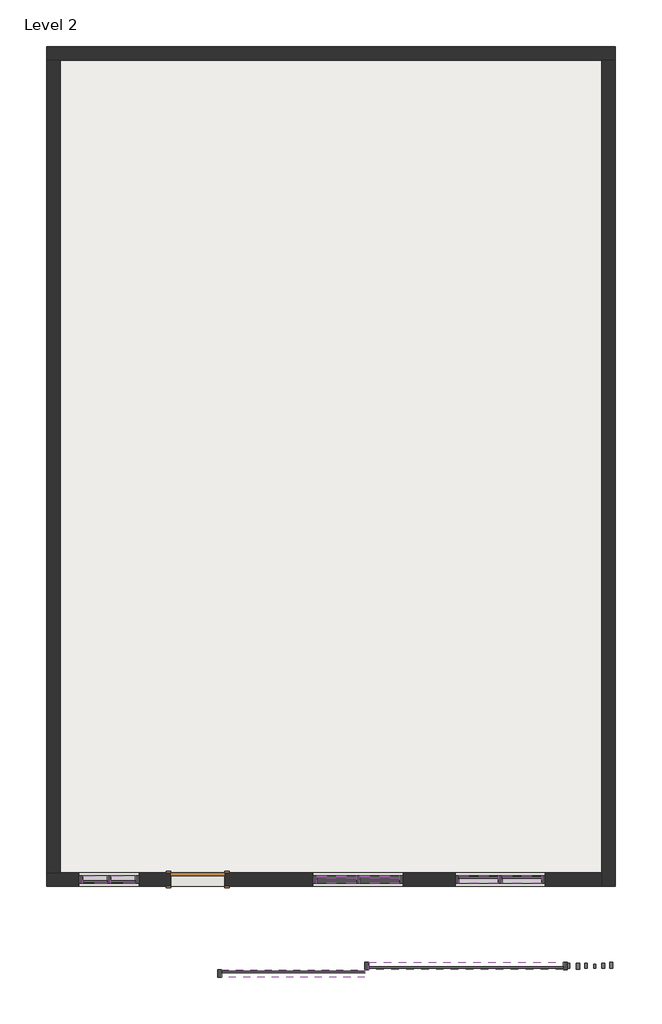
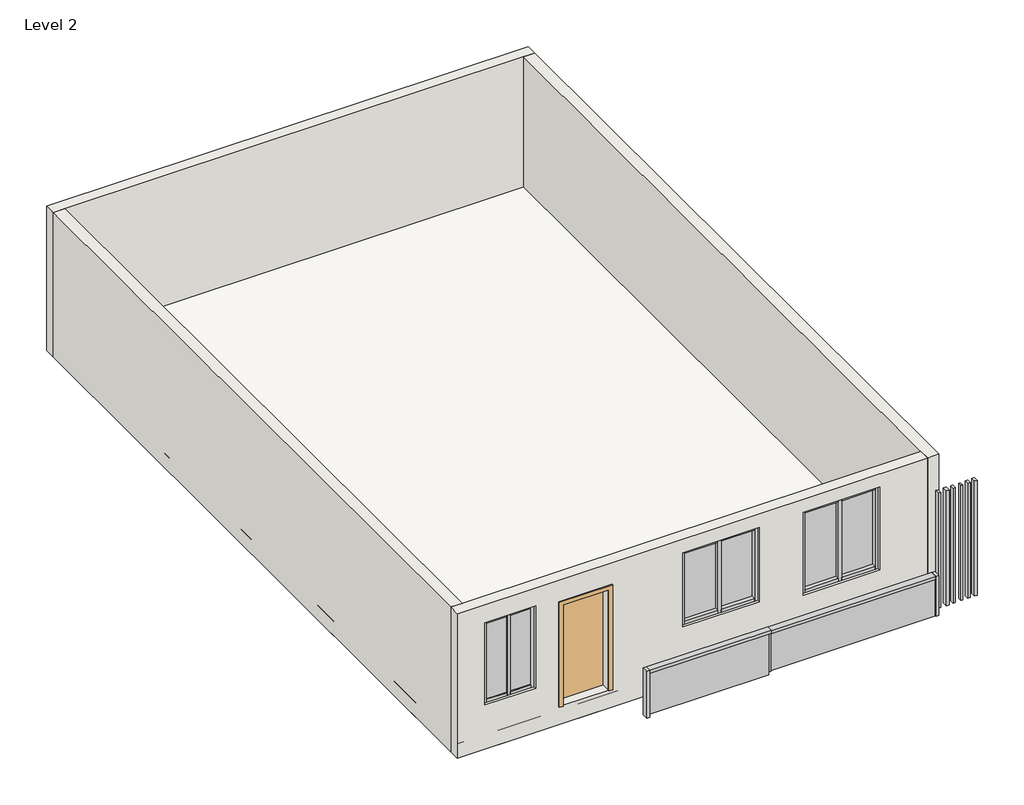
# One storey: 26 members, 8 plates, 4 walls, 1 door, 1 proxy, 1 roof.
"""IFC4 building model written with IfcOpenShell, lengths in millimetres."""

from ifc_helpers import new_model, si_unit, frame, origin, place, context, project, spatial, polyline, outline, extrude, faceted_brep, transform, mapped, element, save
from components import generic_models_4_generic_models_4_fedd3438, door_0ca8825f, member_dc106669, member_8f1d4e4f, member_b289f3f9, member_c33c434a, member_39095dcb, member_2ac6f7d4, member_334bbce8, member_2bb4249f, member_ceefbd1b, member_128fbec0, member_360d9ee7, member_413afe15, system_panel_glazed_02abb1c2, system_panel_glazed_de152a88, system_panel_glazed_dddf758e, system_panel_glazed_6abdcac5, system_panel_glazed_361f77d3

model = new_model("IFC4")

# Units and contexts
model_context = context("Model", 3, world=origin())
ifc_project = project(units=[si_unit("LENGTHUNIT", "METRE", prefix="MILLI")], contexts=[model_context])

# Site, building, storey
site = spatial("IfcSite", under=ifc_project)
building = spatial("IfcBuilding", under=site)
storey = spatial("IfcBuildingStorey", under=building, Name="Level 2", Elevation=3048.0)

# Proxy
placement = place(None, origin())
generic_models_4_generic_models_4_shape = generic_models_4_generic_models_4_fedd3438(model_context)
element("IfcBuildingElementProxy", 1, Name="Generic Models 4 : Generic Models 4", ObjectType="Generic Models 4 : Generic Models 4", at=placement, inside=storey, context=model_context, shape_type="MappedRepresentation", body=[
    mapped(generic_models_4_generic_models_4_shape, transform((0.0, 0.0, 0.0), x_axis=(1.0, 0.0, 0.0), y_axis=(0.0, 1.0, 0.0), z_axis=(0.0, 0.0, 1.0))),
])

# Door
door_shape = door_0ca8825f(model_context)
element("IfcDoor", 2, ObjectType="Single-Flush : 36\" x 84\"", at=placement, inside=storey, context=model_context, shape_type="MappedRepresentation", body=[
    mapped(door_shape, transform((-16080.3094994, -14629.3805842, 3429.0), x_axis=(1.0, 0.0, 0.0), y_axis=(0.0, 1.0, 0.0), z_axis=(0.0, 0.0, 1.0))),
])

# Members
member_shape = member_dc106669(model_context)
element("IfcMember", 3, ObjectType="Rectangular Mullion : 2.5\" x 5\" rectangular", at=placement, inside=storey, context=model_context, shape_type="MappedRepresentation", body=[
    mapped(member_shape, transform((-17610.6594994, -14629.3805842, 3978.3517748), x_axis=(0.0, 0.0, -1.0), y_axis=(0.0, 1.0, 0.0), z_axis=(1.0, 0.0, 0.0))),
])
element("IfcMember", 4, ObjectType="Rectangular Mullion : 2.5\" x 5\" rectangular", at=placement, inside=storey, context=model_context, shape_type="MappedRepresentation", body=[
    mapped(member_shape, transform((-17134.4094994, -14629.3805842, 3978.3517748), x_axis=(0.0, 0.0, -1.0), y_axis=(0.0, 1.0, 0.0), z_axis=(1.0, 0.0, 0.0))),
])
member_2_shape = member_8f1d4e4f(model_context)
element("IfcMember", 5, ObjectType="Rectangular Mullion : 2.5\" x 5\" rectangular", at=placement, inside=storey, context=model_context, shape_type="MappedRepresentation", body=[
    mapped(member_2_shape, transform((-17578.9094994, -14629.3805842, 3978.3517748), x_axis=(-1.0, 0.0, 0.0), y_axis=(0.0, 1.0, 0.0), z_axis=(0.0, 0.0, -1.0))),
])
element("IfcMember", 6, ObjectType="Rectangular Mullion : 2.5\" x 5\" rectangular", at=placement, inside=storey, context=model_context, shape_type="MappedRepresentation", body=[
    mapped(member_shape, transform((-17547.1594994, -14629.3805842, 5711.0482812), x_axis=(0.0, 0.0, 1.0), y_axis=(0.0, 1.0, 0.0), z_axis=(-1.0, 0.0, 0.0))),
])
element("IfcMember", 7, ObjectType="Rectangular Mullion : 2.5\" x 5\" rectangular", at=placement, inside=storey, context=model_context, shape_type="MappedRepresentation", body=[
    mapped(member_shape, transform((-18023.4094994, -14629.3805842, 5711.0482812), x_axis=(0.0, 0.0, 1.0), y_axis=(0.0, 1.0, 0.0), z_axis=(-1.0, 0.0, 0.0))),
])
member_3_shape = member_b289f3f9(model_context)
element("IfcMember", 8, ObjectType="Rectangular Mullion : 2.5\" x 5\" rectangular", at=placement, inside=storey, context=model_context, shape_type="MappedRepresentation", body=[
    mapped(member_3_shape, transform((-18086.9094994, -14629.3805842, 3978.3517748), x_axis=(-1.0, 0.0, 0.0), y_axis=(0.0, 1.0, 0.0), z_axis=(0.0, 0.0, -1.0))),
])
element("IfcMember", 9, ObjectType="Rectangular Mullion : 2.5\" x 5\" rectangular", at=placement, inside=storey, context=model_context, shape_type="MappedRepresentation", body=[
    mapped(member_3_shape, transform((-17070.9094994, -14629.3805842, 5711.0482812), x_axis=(1.0, 0.0, 0.0), y_axis=(0.0, 1.0, 0.0), z_axis=(0.0, 0.0, 1.0))),
])
member_4_shape = member_c33c434a(model_context)
element("IfcMember", 10, ObjectType="Rectangular Mullion : 2.5\" x 5\" rectangular", at=placement, inside=storey, context=model_context, shape_type="MappedRepresentation", body=[
    mapped(member_4_shape, transform((-13343.4594994, -14629.3805842, 4238.4597906), x_axis=(0.0, 0.0, -1.0), y_axis=(0.0, -1.0, 0.0), z_axis=(-1.0, 0.0, 0.0))),
])
element("IfcMember", 11, ObjectType="Rectangular Mullion : 2.5\" x 5\" rectangular", at=placement, inside=storey, context=model_context, shape_type="MappedRepresentation", body=[
    mapped(member_4_shape, transform((-14073.7094994, -14629.3805842, 4238.4597906), x_axis=(0.0, 0.0, -1.0), y_axis=(0.0, -1.0, 0.0), z_axis=(-1.0, 0.0, 0.0))),
])
element("IfcMember", 12, ObjectType="Rectangular Mullion : 2.5\" x 5\" rectangular", at=placement, inside=storey, context=model_context, shape_type="MappedRepresentation", body=[
    mapped(member_4_shape, transform((-10943.1594994, -14629.3805842, 4069.915237), x_axis=(0.0, 0.0, -1.0), y_axis=(0.0, -1.0, 0.0), z_axis=(-1.0, 0.0, 0.0))),
])
element("IfcMember", 13, ObjectType="Rectangular Mullion : 2.5\" x 5\" rectangular", at=placement, inside=storey, context=model_context, shape_type="MappedRepresentation", body=[
    mapped(member_4_shape, transform((-11673.4094994, -14629.3805842, 4069.915237), x_axis=(0.0, 0.0, -1.0), y_axis=(0.0, -1.0, 0.0), z_axis=(-1.0, 0.0, 0.0))),
])
member_5_shape = member_39095dcb(model_context)
element("IfcMember", 14, ObjectType="Rectangular Mullion : 2.5\" x 5\" rectangular", at=placement, inside=storey, context=model_context, shape_type="MappedRepresentation", body=[
    mapped(member_5_shape, transform((-13375.2094994, -14629.3805842, 4238.4597906), x_axis=(1.0, 0.0, 0.0), y_axis=(0.0, -1.0, 0.0), z_axis=(0.0, 0.0, -1.0))),
])
element("IfcMember", 15, ObjectType="Rectangular Mullion : 2.5\" x 5\" rectangular", at=placement, inside=storey, context=model_context, shape_type="MappedRepresentation", body=[
    mapped(member_4_shape, transform((-13406.9594994, -14629.3805842, 5805.439827), x_axis=(0.0, 0.0, 1.0), y_axis=(0.0, -1.0, 0.0), z_axis=(1.0, 0.0, 0.0))),
])
element("IfcMember", 16, ObjectType="Rectangular Mullion : 2.5\" x 5\" rectangular", at=placement, inside=storey, context=model_context, shape_type="MappedRepresentation", body=[
    mapped(member_4_shape, transform((-12676.7094994, -14629.3805842, 5805.439827), x_axis=(0.0, 0.0, 1.0), y_axis=(0.0, -1.0, 0.0), z_axis=(1.0, 0.0, 0.0))),
])
element("IfcMember", 17, ObjectType="Rectangular Mullion : 2.5\" x 5\" rectangular", at=placement, inside=storey, context=model_context, shape_type="MappedRepresentation", body=[
    mapped(member_4_shape, transform((-11006.6594994, -14629.3805842, 5817.9370374), x_axis=(0.0, 0.0, 1.0), y_axis=(0.0, -1.0, 0.0), z_axis=(1.0, 0.0, 0.0))),
])
element("IfcMember", 18, ObjectType="Rectangular Mullion : 2.5\" x 5\" rectangular", at=placement, inside=storey, context=model_context, shape_type="MappedRepresentation", body=[
    mapped(member_4_shape, transform((-10276.4094994, -14629.3805842, 5817.9370374), x_axis=(0.0, 0.0, 1.0), y_axis=(0.0, -1.0, 0.0), z_axis=(1.0, 0.0, 0.0))),
])
member_6_shape = member_2ac6f7d4(model_context)
element("IfcMember", 19, ObjectType="Rectangular Mullion : 2.5\" x 5\" rectangular", at=placement, inside=storey, context=model_context, shape_type="MappedRepresentation", body=[
    mapped(member_6_shape, transform((-14137.2094994, -14629.3805842, 5805.439827), x_axis=(-1.0, 0.0, 0.0), y_axis=(0.0, -1.0, 0.0), z_axis=(0.0, 0.0, 1.0))),
])
element("IfcMember", 20, ObjectType="Rectangular Mullion : 2.5\" x 5\" rectangular", at=placement, inside=storey, context=model_context, shape_type="MappedRepresentation", body=[
    mapped(member_6_shape, transform((-12613.2094994, -14629.3805842, 4238.4597906), x_axis=(1.0, 0.0, 0.0), y_axis=(0.0, -1.0, 0.0), z_axis=(0.0, 0.0, -1.0))),
])
member_7_shape = member_334bbce8(model_context)
element("IfcMember", 21, ObjectType="Rectangular Mullion : 2.5\" x 5\" rectangular", at=placement, inside=storey, context=model_context, shape_type="MappedRepresentation", body=[
    mapped(member_7_shape, transform((-10974.9094994, -14629.3805842, 4069.915237), x_axis=(1.0, 0.0, 0.0), y_axis=(0.0, -1.0, 0.0), z_axis=(0.0, 0.0, -1.0))),
])
member_8_shape = member_2bb4249f(model_context)
element("IfcMember", 22, ObjectType="Rectangular Mullion : 2.5\" x 5\" rectangular", at=placement, inside=storey, context=model_context, shape_type="MappedRepresentation", body=[
    mapped(member_8_shape, transform((-11736.9094994, -14629.3805842, 5817.9370374), x_axis=(-1.0, 0.0, 0.0), y_axis=(0.0, -1.0, 0.0), z_axis=(0.0, 0.0, 1.0))),
])
element("IfcMember", 23, ObjectType="Rectangular Mullion : 2.5\" x 5\" rectangular", at=placement, inside=storey, context=model_context, shape_type="MappedRepresentation", body=[
    mapped(member_8_shape, transform((-10212.9094994, -14629.3805842, 4069.915237), x_axis=(1.0, 0.0, 0.0), y_axis=(0.0, -1.0, 0.0), z_axis=(0.0, 0.0, -1.0))),
])
member_9_shape = member_ceefbd1b(model_context)
element("IfcMember", 24, ObjectType="Rectangular Mullion : 2.5\" x 5\" rectangular", at=placement, inside=storey, context=model_context, shape_type="MappedRepresentation", body=[
    mapped(member_9_shape, transform((-13260.9094994, -16086.1836279, 3832.9773714), x_axis=(-1.0, 0.0, 0.0), y_axis=(0.0, 1.0, 0.0), z_axis=(0.0, 0.0, -1.0))),
])
member_10_shape = member_128fbec0(model_context)
element("IfcMember", 25, ObjectType="Rectangular Mullion : 2.5\" x 5\" rectangular", at=placement, inside=storey, context=model_context, shape_type="MappedRepresentation", body=[
    mapped(member_10_shape, transform((-13197.4094994, -16086.1836279, 4684.2815968), x_axis=(0.0, 0.0, 1.0), y_axis=(0.0, 1.0, 0.0), z_axis=(-1.0, 0.0, 0.0))),
])
element("IfcMember", 26, ObjectType="Rectangular Mullion : 2.5\" x 5\" rectangular", at=placement, inside=storey, context=model_context, shape_type="MappedRepresentation", body=[
    mapped(member_9_shape, transform((-9847.8329873, -16086.1836279, 4684.2815968), x_axis=(1.0, 0.0, 0.0), y_axis=(0.0, 1.0, 0.0), z_axis=(0.0, 0.0, 1.0))),
])
member_11_shape = member_360d9ee7(model_context)
element("IfcMember", 27, ObjectType="Rectangular Mullion : 2.5\" x 5\" rectangular", at=placement, inside=storey, context=model_context, shape_type="MappedRepresentation", body=[
    mapped(member_11_shape, transform((-13260.9094994, -16218.2200166, 4795.8020734), x_axis=(0.0, 0.0, 1.0), y_axis=(0.0, -1.0, 0.0), z_axis=(1.0, 0.0, 0.0))),
])
member_12_shape = member_413afe15(model_context)
element("IfcMember", 28, ObjectType="Rectangular Mullion : 2.5\" x 5\" rectangular", at=placement, inside=storey, context=model_context, shape_type="MappedRepresentation", body=[
    mapped(member_12_shape, transform((-15742.353759, -16218.2200166, 4795.8020734), x_axis=(-1.0, 0.0, 0.0), y_axis=(0.0, -1.0, 0.0), z_axis=(0.0, 0.0, 1.0))),
])

# Plates
system_panel_glazed_shape = system_panel_glazed_02abb1c2(model_context)
element("IfcPlate", 29, ObjectType="System Panel : Glazed", at=placement, inside=storey, context=model_context, shape_type="MappedRepresentation", body=[
    mapped(system_panel_glazed_shape, transform((-17340.7844994, -14629.3805842, 4041.8517748), x_axis=(-1.0, 0.0, 0.0), y_axis=(0.0, -1.0, 0.0), z_axis=(0.0, 0.0, 1.0))),
])
element("IfcPlate", 30, ObjectType="System Panel : Glazed", at=placement, inside=storey, context=model_context, shape_type="MappedRepresentation", body=[
    mapped(system_panel_glazed_shape, transform((-17817.0344994, -14629.3805842, 4041.8517748), x_axis=(-1.0, 0.0, 0.0), y_axis=(0.0, -1.0, 0.0), z_axis=(0.0, 0.0, 1.0))),
])
system_panel_glazed_2_shape = system_panel_glazed_de152a88(model_context)
element("IfcPlate", 31, ObjectType="System Panel : Glazed", at=placement, inside=storey, context=model_context, shape_type="MappedRepresentation", body=[
    mapped(system_panel_glazed_2_shape, transform((-13740.3344994, -14629.3805842, 4301.9597906), x_axis=(1.0, 0.0, 0.0), y_axis=(0.0, 1.0, 0.0), z_axis=(0.0, 0.0, 1.0))),
])
element("IfcPlate", 32, ObjectType="System Panel : Glazed", at=placement, inside=storey, context=model_context, shape_type="MappedRepresentation", body=[
    mapped(system_panel_glazed_2_shape, transform((-13010.0844994, -14629.3805842, 4301.9597906), x_axis=(1.0, 0.0, 0.0), y_axis=(0.0, 1.0, 0.0), z_axis=(0.0, 0.0, 1.0))),
])
system_panel_glazed_3_shape = system_panel_glazed_dddf758e(model_context)
element("IfcPlate", 33, ObjectType="System Panel : Glazed", at=placement, inside=storey, context=model_context, shape_type="MappedRepresentation", body=[
    mapped(system_panel_glazed_3_shape, transform((-11340.0344994, -14629.3805842, 4133.415237), x_axis=(1.0, 0.0, 0.0), y_axis=(0.0, 1.0, 0.0), z_axis=(0.0, 0.0, 1.0))),
])
element("IfcPlate", 34, ObjectType="System Panel : Glazed", at=placement, inside=storey, context=model_context, shape_type="MappedRepresentation", body=[
    mapped(system_panel_glazed_3_shape, transform((-10609.7844994, -14629.3805842, 4133.415237), x_axis=(1.0, 0.0, 0.0), y_axis=(0.0, 1.0, 0.0), z_axis=(0.0, 0.0, 1.0))),
])
system_panel_glazed_4_shape = system_panel_glazed_6abdcac5(model_context)
element("IfcPlate", 35, ObjectType="System Panel : Glazed", at=placement, inside=storey, context=model_context, shape_type="MappedRepresentation", body=[
    mapped(system_panel_glazed_4_shape, transform((-11554.3712434, -16086.1836279, 3832.9773714), x_axis=(-1.0, 0.0, 0.0), y_axis=(0.0, -1.0, 0.0), z_axis=(0.0, 0.0, 1.0))),
])
system_panel_glazed_5_shape = system_panel_glazed_361f77d3(model_context)
element("IfcPlate", 36, ObjectType="System Panel : Glazed", at=placement, inside=storey, context=model_context, shape_type="MappedRepresentation", body=[
    mapped(system_panel_glazed_5_shape, transform((-14469.8816292, -16218.2200166, 3811.3624223), x_axis=(1.0, 0.0, 0.0), y_axis=(0.0, 1.0, 0.0), z_axis=(0.0, 0.0, 1.0))),
])

# Roof
element("IfcRoof", 37, ObjectType="Generic - 12\"", at=placement, inside=storey, context=model_context, shape_type="SweptSolid", body=[
    extrude(outline(polyline([(-18633.0094994, -570.4805842), (-9031.8094994, -570.4805842), (-9031.8094994, -14743.6805842), (-18633.0094994, -14743.6805842), (-18633.0094994, -570.4805842)])), frame((0.0, 0.0, 3048.0), z_axis=(0.0, 0.0, 1.0), x_axis=(1.0, 0.0, 0.0)), (0.0, 0.0, 1.0), 304.8),
])

# Walls
element("IfcWall", 38, ObjectType="9\"", at=placement, inside=storey, context=model_context, shape_type="Brep", body=[
    faceted_brep([(-18633.0094994, -799.0805842, 3048.0), (-18404.4094994, -799.0805842, 3048.0), (-9260.4094994, -799.0805842, 3048.0), (-9031.8094994, -799.0805842, 3048.0), (-9031.8094994, -799.0805842, 6096.0), (-9260.4094994, -799.0805842, 6096.0), (-18404.4094994, -799.0805842, 6096.0), (-18633.0094994, -799.0805842, 6096.0), (-18633.0094994, -570.4805842, 3048.0), (-18633.0094994, -570.4805842, 6096.0), (-9031.8094994, -570.4805842, 6096.0), (-9031.8094994, -570.4805842, 3048.0)], [[[0, 1, 2, 3, 4, 5, 6, 7]], [[8, 9, 10, 11]], [[3, 2, 1, 0, 8, 11]], [[7, 6, 5, 4, 10, 9]], [[4, 3, 11, 10]], [[0, 7, 9, 8]]]),
])
element("IfcWall", 39, ObjectType="9\"", at=placement, inside=storey, context=model_context, shape_type="Brep", body=[
    faceted_brep([(-9260.4094994, -799.0805842, 3048.0), (-9260.4094994, -14515.0805842, 3048.0), (-9260.4094994, -14743.6805842, 3048.0), (-9260.4094994, -14743.6805842, 6096.0), (-9260.4094994, -14515.0805842, 6096.0), (-9260.4094994, -799.0805842, 6096.0), (-9031.8094994, -799.0805842, 3048.0), (-9031.8094994, -799.0805842, 6096.0), (-9031.8094994, -14743.6805842, 6096.0), (-9031.8094994, -14743.6805842, 3048.0)], [[[0, 1, 2, 3, 4, 5]], [[6, 7, 8, 9]], [[2, 1, 0, 6, 9]], [[5, 4, 3, 8, 7]], [[0, 5, 7, 6]], [[3, 2, 9, 8]]]),
])
element("IfcWall", 40, ObjectType="9\"", at=placement, inside=storey, context=model_context, shape_type="Brep", body=[
    faceted_brep([(-9260.4094994, -14515.0805842, 3048.0), (-18404.4094994, -14515.0805842, 3048.0), (-18633.0094994, -14515.0805842, 3048.0), (-18633.0094994, -14515.0805842, 6096.0), (-18404.4094994, -14515.0805842, 6096.0), (-9260.4094994, -14515.0805842, 6096.0), (-16537.5094994, -14515.0805842, 3429.0), (-15623.1094994, -14515.0805842, 3429.0), (-15623.1094994, -14515.0805842, 5562.6), (-16537.5094994, -14515.0805842, 5562.6), (-17070.9094994, -14515.0805842, 3978.3517748), (-17070.9094994, -14515.0805842, 5711.0482812), (-18086.9094994, -14515.0805842, 5711.0482812), (-18086.9094994, -14515.0805842, 3978.3517748), (-14137.2094994, -14515.0805842, 5805.439827), (-14137.2094994, -14515.0805842, 4238.4597906), (-12613.2094994, -14515.0805842, 4238.4597906), (-12613.2094994, -14515.0805842, 5805.439827), (-11736.9094994, -14515.0805842, 5817.9370374), (-11736.9094994, -14515.0805842, 4069.915237), (-10212.9094994, -14515.0805842, 4069.915237), (-10212.9094994, -14515.0805842, 5817.9370374), (-18633.0094994, -14743.6805842, 3048.0), (-9260.4094994, -14743.6805842, 3048.0), (-9260.4094994, -14743.6805842, 6096.0), (-18633.0094994, -14743.6805842, 6096.0), (-15623.1094994, -14743.6805842, 3429.0), (-16537.5094994, -14743.6805842, 3429.0), (-16537.5094994, -14743.6805842, 5562.6), (-15623.1094994, -14743.6805842, 5562.6), (-17070.9094994, -14743.6805842, 5711.0482812), (-17070.9094994, -14743.6805842, 3978.3517748), (-18086.9094994, -14743.6805842, 3978.3517748), (-18086.9094994, -14743.6805842, 5711.0482812), (-14137.2094994, -14743.6805842, 4238.4597906), (-14137.2094994, -14743.6805842, 5805.439827), (-12613.2094994, -14743.6805842, 5805.439827), (-12613.2094994, -14743.6805842, 4238.4597906), (-11736.9094994, -14743.6805842, 4069.915237), (-11736.9094994, -14743.6805842, 5817.9370374), (-10212.9094994, -14743.6805842, 5817.9370374), (-10212.9094994, -14743.6805842, 4069.915237)], [[[0, 1, 2, 3, 4, 5], [6, 7, 8, 9], [10, 11, 12, 13], [14, 15, 16, 17], [18, 19, 20, 21]], [[22, 23, 24, 25], [26, 27, 28, 29], [30, 31, 32, 33], [34, 35, 36, 37], [38, 39, 40, 41]], [[2, 1, 0, 23, 22]], [[5, 4, 3, 25, 24]], [[0, 5, 24, 23]], [[3, 2, 22, 25]], [[7, 6, 27, 26]], [[8, 7, 26, 29]], [[9, 8, 29, 28]], [[6, 9, 28, 27]], [[30, 11, 10, 31]], [[11, 30, 33, 12]], [[12, 33, 32, 13]], [[31, 10, 13, 32]], [[34, 15, 14, 35]], [[35, 14, 17, 36]], [[36, 17, 16, 37]], [[15, 34, 37, 16]], [[18, 39, 38, 19]], [[39, 18, 21, 40]], [[40, 21, 20, 41]], [[19, 38, 41, 20]]]),
])
element("IfcWall", 41, ObjectType="9\"", at=placement, inside=storey, context=model_context, shape_type="SweptSolid", body=[
    extrude(outline(polyline([(-18633.0094994, -14515.0805842), (-18633.0094994, -799.0805842), (-18404.4094994, -799.0805842), (-18404.4094994, -14515.0805842), (-18633.0094994, -14515.0805842)])), frame((0.0, 0.0, 3048.0), z_axis=(0.0, 0.0, 1.0), x_axis=(1.0, 0.0, 0.0)), (0.0, 0.0, 1.0), 3048.0),
])

save(model, "model.ifc")

# Revit data of these elements
# Type "Single-Flush : 36\" x 84\""
#   Type Mark = "1"
#   Construction Type Id = "MDOOR"
#   Assembly Code = "C1020"
#   Analytic Construction = "Metal"
#   Thickness = 0' - 2"
#   Heat Transfer Coefficient (U) = 0.651978 BTU/(h·ft²·°F)
#   Height = 7' - 0"
#   Trim Projection Ext = 0' - 1"
#   Trim Projection Int = 0' - 1"
#   Trim Width = 0' - 3"
#   Width = 3' - 0"
#   Define Thermal Properties by = 1
#   Define Thermal Properties by = 1
#   Door Material = Door - Panel
#   Frame Material = Door - Frame
#   Visual Light Transmittance = 0
#   Solar Heat Gain Coefficient = 0
#   Function = (empty or 0)
#   Wall Closure = (empty or 0)
# Type "Rectangular Mullion : 2.5\" x 5\" rectangular"
#   built-in parameter 1007304 = 0.416667 (stored number, unit not read)
#   built-in parameter 1007301 = 0.104167 (stored number, unit not read)
#   built-in parameter 1007300 = 0.104167 (stored number, unit not read)
# Type "System Panel : Glazed"
#   Construction Type Id = "GSP4R"
#   Analytic Construction = "1/8 in Pilkington single glazing"
#   Visual Light Transmittance = 0.9
#   Solar Heat Gain Coefficient = 0.86
#   Heat Transfer Coefficient (U) = 1.18115 BTU/(h·ft²·°F)
#   Define Thermal Properties by = 1
# Type "Generic - 12\""
#   Assembly Code = "B1020"
#   Layers, outside or top first: 1' - 0" no material (function 1)
# Type "9\""
#   Assembly Code = "B2010"
#   Layers, outside or top first: 0' - 9" no material (function 1)
# Element 1 (IfcBuildingElementProxy, "Generic Models 4 : Generic Models 4")
#   Phase Created = New Construction
# Element 2 (IfcDoor, "Single-Flush : 36\" x 84\"")
#   Phase Created = New Construction
#   Materials on its faces: "Door - Frame", "Door - Panel"
# Elements 3, 4, 5, 6, 7, 8, 9, 10, 11, 12, 13, 14, 15, 16, 17, 18, 19, 20, 21, 22, 23, 24, 25, 26, 27, 28 (IfcMember, "Rectangular Mullion : 2.5\" x 5\" rectangular")
#   Phase Created = New Construction
#   Materials on its faces: "Aluminum"
# Elements 29, 30, 31, 32, 33, 34, 35, 36 (IfcPlate, "System Panel : Glazed")
#   Phase Created = New Construction
#   Materials on its faces: "Glass"
# Element 37 (IfcRoof, "Generic - 12\"")
#   built-in parameter 1001705 = 11 (stored number, unit not read)
#   built-in parameter 1001710 = 33615
#   Phase Created = New Construction
#   Materials on its faces: "Default Roof"
# Elements 38, 39, 40, 41 (IfcWall, "9\"")
#   Top Offset = 0' - 0"
#   Base Offset = 0' - 0"
#   Unconnected Height = 10' - 0"
#   wall height = 10' - 0"
#   Phase Created = New Construction
#   Base Constraint = Level 2
#   Materials on its faces: "Default Wall"
# Materials
#   "Door - Panel": class "Wood", colour RGB 210 159 95, transparency 0, Cost = 0
#   "Door - Frame": colour RGB 118 70 51, transparency 0, Cost = 0
#   "Aluminum": class "Metal", colour RGB 247 247 247, transparency 0, Description = "Aluminum 6061", Cost = 0
#   "Glass": class "Glass", colour RGB 0 128 192, transparency 0.75, Description = "Soda Lime Glass", Cost = 0
#   "Default Roof": colour RGB 88 101 114, transparency 0, Cost = 0
#   "Default Wall": colour RGB 128 128 128, transparency 0, Cost = 0
